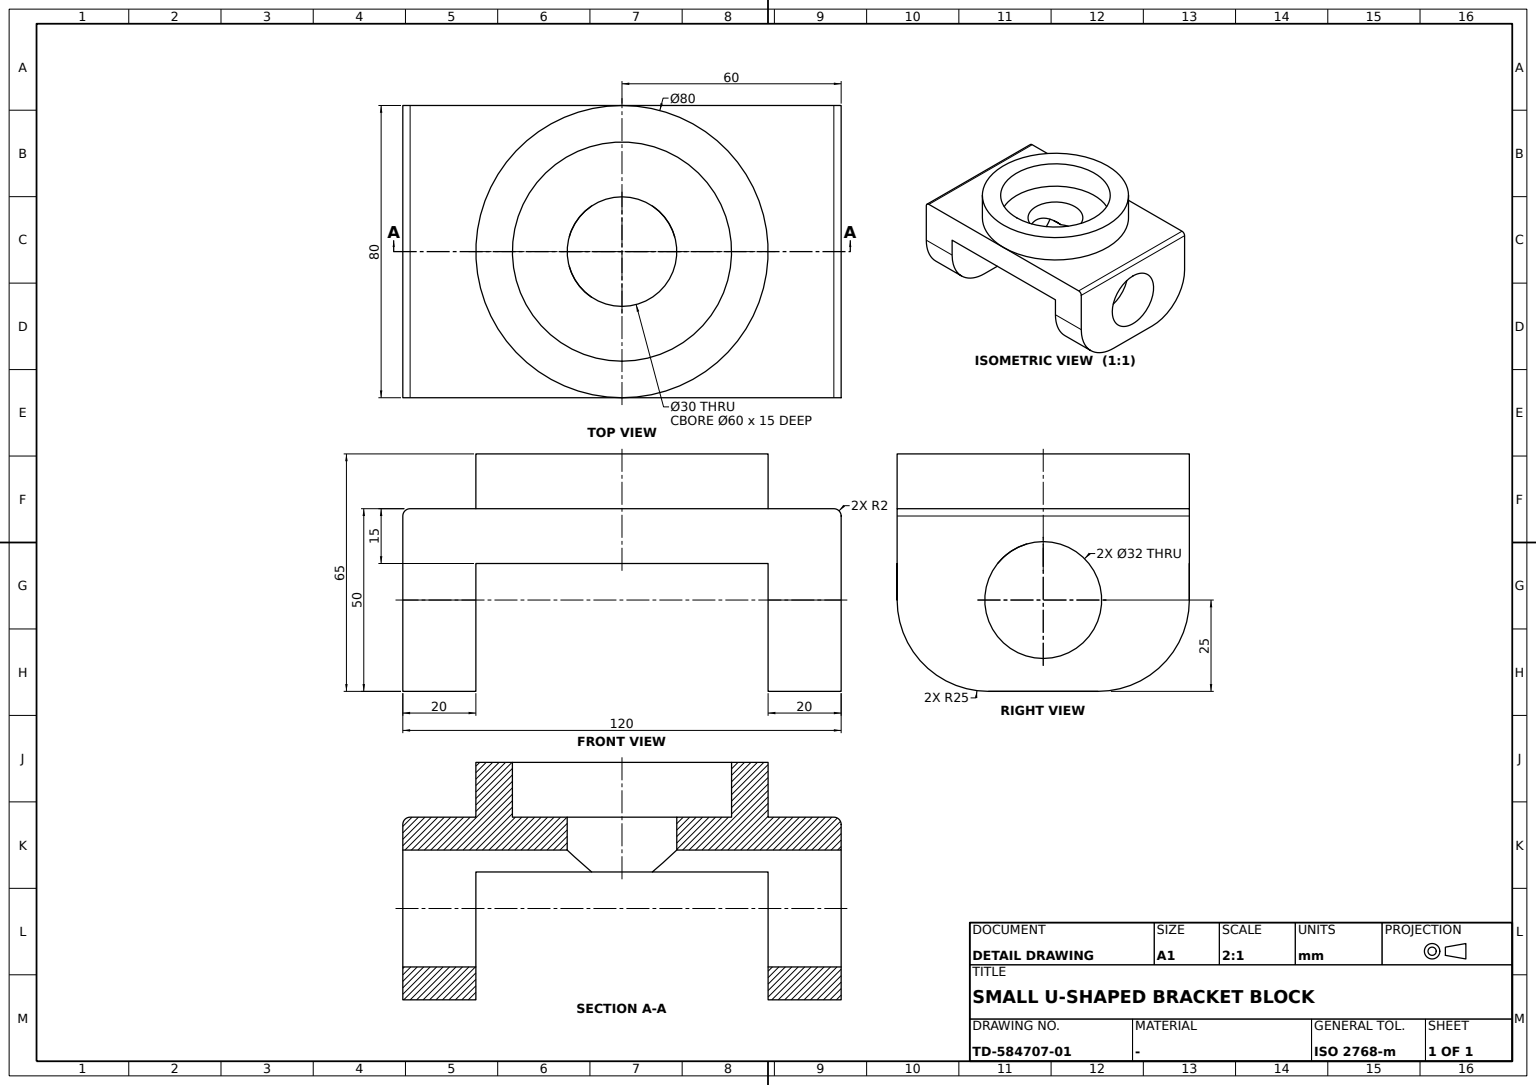
CATIA V5 part; units mm, degrees
sketch "Sketch1" plane through (0, 0, 0) normal (1, 0, 0) x (0, 1, 0)
  line L0 (-40, -35) -> (-40, 0)
  point P0 (-40, 0)
  line L1 (-40, 0) -> (40, 0)
  line L2 (40, 0) -> (40, -35)
  line L3 (40, -35) -> (60, -35)
  line L4 (60, -35) -> (60, 15)
  line L5 (60, 15) -> (-60, 15)
  line L6 (-60, 15) -> (-60, -35)
  point P1 (-60, -35)
  line L7 (-60, -35) -> (-40, -35)
  dimension "length L4" = 50
  dimension "distance L5 x axis" = 15
  dimension "length L7" = 20
  dimension "length L3" = 20
  dimension "length L1" = 80
  constraint coincidence P0 x-axis
  constraint coincidence P1 L3
  constraint vertical L0 y-axis
  constraint vertical L2 y-axis
  constraint vertical L4 y-axis
  constraint vertical L6 y-axis
  constraint horizontal L1 x-axis
  constraint horizontal L3 x-axis
  constraint horizontal L5 x-axis
  constraint horizontal L7 x-axis
  constraint symmetry L4 L6 y-axis
extrude "Pad1" add sketch "Sketch1" along normal mid plane 80
ref_plane "Plane1" through (0, 0, 15) normal (0, 0, 1) x (1, 0, 0)
sketch "Sketch2" plane through (0, 0, 15) normal (0, 0, 1) x (1, 0, 0)
  circle A0 centre (0, 0) radius 30
  circle A1 centre (0, 0) radius 40
  dimension "radius A1" = 40
  dimension "radius A0" = 30
extrude "Pad2" add sketch "Sketch2" along normal blind 15
sketch "Sketch3" plane through (0, 0, 15) normal (0, 0, 1) x (1, 0, 0)
  circle A0 centre (0, 0) radius 15
  dimension "radius A0" = 15
extrude "Pocket1" cut sketch "Sketch3" against normal blind 15
sketch "Sketch4" plane through (0, 60, 0) normal (0, 1, 0) x (-1, 0, 0)
  circle A0 centre (0, -10) radius 16
  point P0 (0, -10)
  line L0 (40, -35) -> (-40, -35) construction
  dimension "distance P0 L0" = 25
  dimension "radius A0" = 16
  constraint coincidence P0 y-axis
extrude "Pocket2" cut sketch "Sketch4" against normal through all
fillet "Fillet1" radius 25 1 edges at (40, 50, -35)
fillet "Fillet2" radius 25 1 edges at (-40, 50, -35)
fillet "Fillet3" radius 25 1 edges at (-40, -50, -35)
fillet "Fillet4" radius 25 1 edges at (40, -50, -35)
fillet "Fillet5" radius 2 1 edges at (0, -60, 15)
fillet "Fillet6" radius 2 1 edges at (0, 60, 15)
